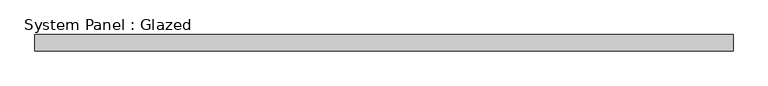
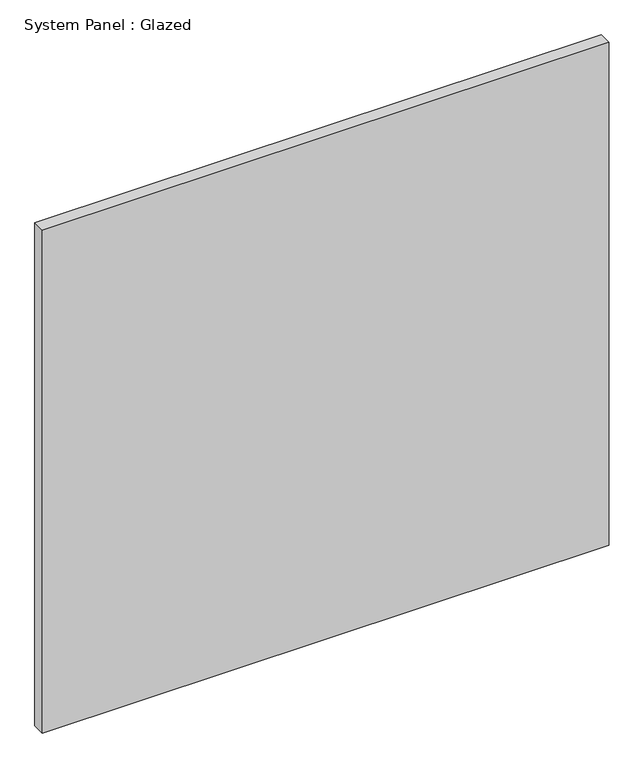
"""IFC4 building model written with IfcOpenShell, lengths in millimetres: plate geometry, System Panel : Glazed."""

from ifc_helpers import new_model, si_unit, origin, origin_with_axes, place, context, project, spatial, polyline, outline, extrude, source, transform, mapped, element, save


def system_panel_glazed_533eadb3(model_context):
    return source(origin(), model_context, "Body", "SweptSolid", [
        extrude(outline(polyline([(549.2750001, 19.05), (-549.2750001, 19.05), (-549.2750001, 44.45), (549.2750001, 44.45), (549.2750001, 19.05)])), origin_with_axes(), (0.0, 0.0, 1.0), 1030.2424454),
    ])


if __name__ == "__main__":
    model = new_model("IFC4")
    model_context = context("Model", 3, world=origin())
    ifc_project = project(units=[si_unit("LENGTHUNIT", "METRE", prefix="MILLI")], contexts=[model_context])
    site = spatial("IfcSite", under=ifc_project)
    building = spatial("IfcBuilding", under=site)
    placement = place(None, origin())
    system_panel_glazed_shape = system_panel_glazed_533eadb3(model_context)
    element("IfcPlate", 1, ObjectType="System Panel : Glazed", at=placement, inside=building, context=model_context, shape_type="MappedRepresentation", body=[
        mapped(system_panel_glazed_shape, transform((0.0, 0.0, 0.0), x_axis=(1.0, 0.0, 0.0), y_axis=(0.0, 1.0, 0.0), z_axis=(0.0, 0.0, 1.0))),
    ])
    save(model, "model.ifc")

# Revit data of these elements
# Type "System Panel : Glazed"
#   Construction Type Id = "GSP4R"
#   Analytic Construction = "1/8 in Pilkington single glazing"
#   Visual Light Transmittance = 0.9
#   Solar Heat Gain Coefficient = 0.86
#   Heat Transfer Coefficient (U) = 1.18115 BTU/(h·ft²·°F)
#   Define Thermal Properties by = 1
# Element 1 (IfcPlate, "System Panel : Glazed")
#   Materials on its faces: "Glass"
# Materials
#   "Glass": class "Glass", colour RGB 0 128 192, transparency 0.75, Description = "Soda Lime Glass", Cost = 0
